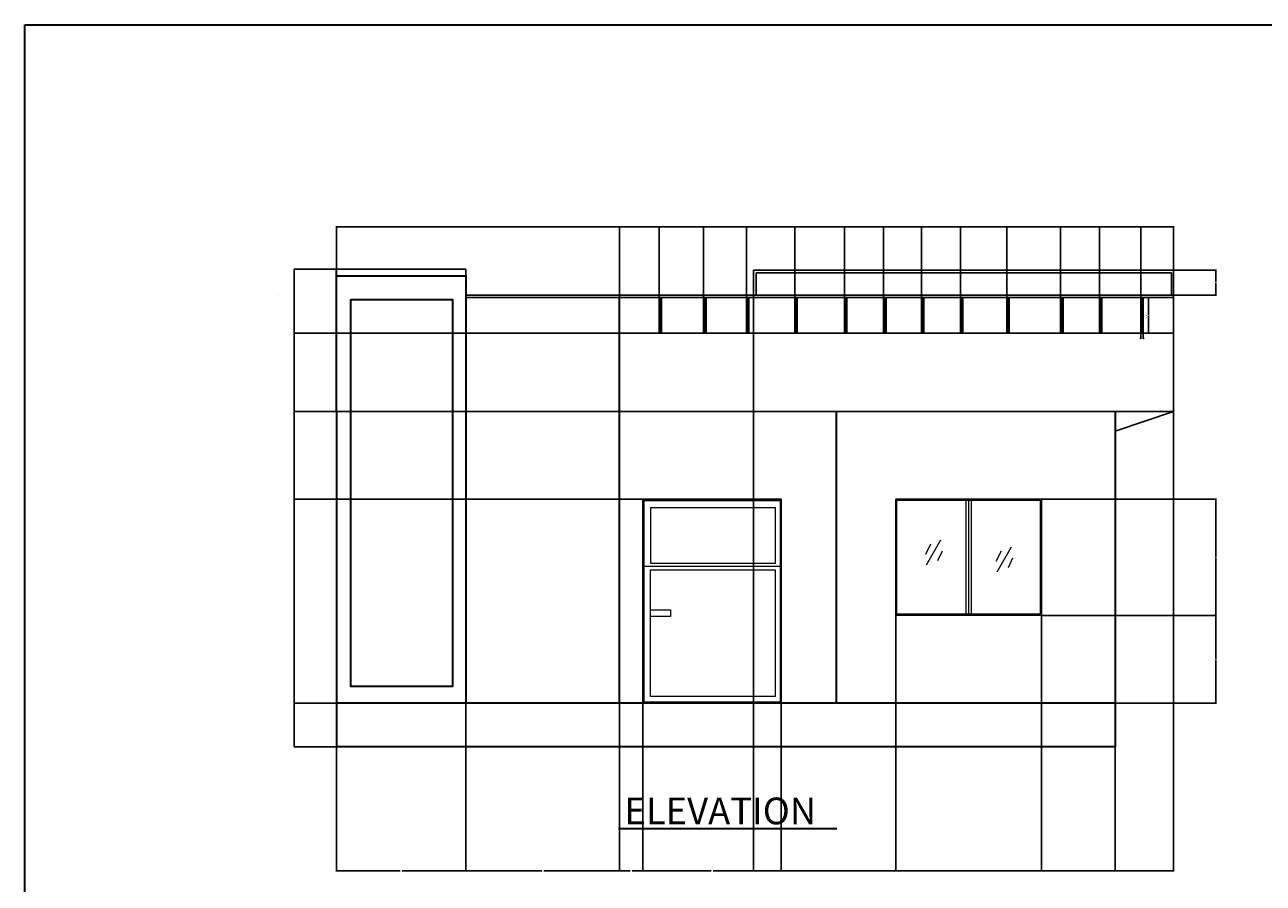
# Model space of a CAD drawing. Units: inches. Extents: x 1441 to 2460, y 1648 to 2683.
# Tile 34 of 35: x 1441 to 1950, y 2329 to 2683. Entities that reach past the tile are written whole.
import ezdxf

# ---------------------------------------------------------------- set-up
doc = ezdxf.new("R2010")
doc.units = ezdxf.units.IN
for name, color, linetype, lineweight in [('A-ANNO-DIMS', 2, 'Continuous', 18), ('A-ANNO-TITL', 7, 'Continuous', 30), ('A-ANNO-TTLB', 7, 'Continuous', 35), ('A-ELEV', 7, 'Continuous', 30), ('A-ELEV-DOOR', 3, 'Continuous', 20), ('A-ELEV-GLAZ', 4, 'Continuous', 18), ('A-ROOF', 7, 'Continuous', 25)]:
    doc.layers.add(name, color=color, linetype=linetype, lineweight=lineweight)
doc.styles.get("Standard").update_dxf_attribs({"font": 'arial.ttf'})
doc.dimstyles.get("Standard").update_dxf_attribs({"dimtxt": 0.18, "dimasz": 0.18, "dimexe": 0.18, "dimexo": 0.0625, "dimgap": 0.09, "dimtad": 0, "dimtih": 1, "dimtoh": 1, "dimdec": 4, "dimzin": 0, "dimdsep": 46, "dimtxsty": 'Standard', "dimcen": 0.09, "dimadec": 0, "dimazin": 0, "dimtfac": 1, "dimtdec": 4, "dimtofl": 0, "dimtmove": 0, "dimatfit": 3, "dimfxl": 1, "dimtolj": 1, "dimtzin": 0, "dimarcsym": 0})

# ---------------------------------------------------------------- blocks, each defined once
blk = doc.blocks.new('PARAPET-MULLION-ELEV')
for p, q in [((0, 14.7), (0, 0)), ((0.5, 0), (0.5, 14.7)), ((1, 14.7), (1, 0))]:
    blk.add_line(p, q)
blk = doc.blocks.new('*D64')
at = {"layer": 'A-ANNO-DIMS', "color": 0, "lineweight": -2, "transparency": 16777216}
for p, q in [((1900.97, 2570.36), (1903.29, 2570.36)), ((1903.11, 2570.18), (1903.11, 2563.2)), ((1903.11, 2555.84), (1903.11, 2562.83)), ((1900.97, 2555.66), (1903.29, 2555.66))]:
    blk.add_line(p, q, dxfattribs=at)
at = {"layer": 'A-ANNO-DIMS', "color": 0, "transparency": 16777216}
for points in [[(1903.08, 2570.18), (1903.14, 2570.18), (1903.11, 2570.36)], [(1903.08, 2555.84), (1903.14, 2555.84), (1903.11, 2555.66)]]:
    blk.add_solid(points, dxfattribs=at)
at = {"layer": 'Defpoints', "color": 0, "transparency": 16777216}
for p in [(1900.91, 2570.36), (1903.11, 2570.36), (1900.91, 2555.66)]:
    blk.add_point(p, dxfattribs=at)
at = {"layer": 'A-ANNO-DIMS', "color": 0, "transparency": 16777216, "insert": (1903.11, 2563.01), "char_height": 0.18, "attachment_point": 5}
blk.add_mtext('\\A1;MULLION 15 TYP.', dxfattribs=at)
blk = doc.blocks.new('*D65')
at = {"layer": 'A-ANNO-DIMS', "color": 0, "lineweight": -2, "transparency": 16777216}
for p, q in [((1899.91, 2555.6), (1899.91, 2553.28)), ((1900.91, 2555.6), (1900.91, 2553.28)), ((1899.73, 2553.46), (1899.55, 2553.46)), ((1901.09, 2553.46), (1901.27, 2553.46))]:
    blk.add_line(p, q, dxfattribs=at)
at = {"layer": 'A-ANNO-DIMS', "color": 0, "transparency": 16777216}
for points in [[(1899.73, 2553.49), (1899.73, 2553.43), (1899.91, 2553.46)], [(1901.09, 2553.49), (1901.09, 2553.43), (1900.91, 2553.46)]]:
    blk.add_solid(points, dxfattribs=at)
at = {"layer": 'Defpoints', "color": 0, "transparency": 16777216}
for p in [(1899.91, 2555.66), (1900.91, 2555.66), (1900.91, 2553.46)]:
    blk.add_point(p, dxfattribs=at)
at = {"layer": 'A-ANNO-DIMS', "color": 0, "transparency": 16777216, "insert": (1900.41, 2553.46), "char_height": 0.18, "attachment_point": 5}
blk.add_mtext('\\A1;1 TYP.', dxfattribs=at)
blk = doc.blocks.new('*D90')
at = {"layer": 'A-ANNO-DIMS', "color": 0, "lineweight": -2, "transparency": 16777216}
for p, q in [((1568.89, 2582.04), (1568.89, 2599.66)), ((1569.07, 2599.48), (1740.74, 2599.48)), ((1913.21, 2599.48), (1741.53, 2599.48)), ((1913.39, 2581.67), (1913.39, 2599.66))]:
    blk.add_line(p, q, dxfattribs=at)
at = {"layer": 'A-ANNO-DIMS', "color": 0, "transparency": 16777216}
for points in [[(1569.07, 2599.51), (1569.07, 2599.45), (1568.89, 2599.48)], [(1913.21, 2599.51), (1913.21, 2599.45), (1913.39, 2599.48)]]:
    blk.add_solid(points, dxfattribs=at)
at = {"layer": 'Defpoints', "color": 0, "transparency": 16777216}
for p in [(1913.39, 2599.48), (1568.89, 2581.98), (1913.39, 2581.61)]:
    blk.add_point(p, dxfattribs=at)
at = {"layer": 'A-ANNO-DIMS', "color": 0, "transparency": 16777216, "insert": (1741.14, 2599.48), "char_height": 0.18, "attachment_point": 5}
blk.add_mtext('\\A1;344.5', dxfattribs=at)
blk = doc.blocks.new('*D91')
at = {"layer": 'A-ANNO-DIMS', "color": 0, "lineweight": -2, "transparency": 16777216}
for p, q in [((1568.82, 2581.98), (1551.21, 2581.98)), ((1551.39, 2581.8), (1551.39, 2483.85)), ((1551.39, 2385.54), (1551.39, 2483.49)), ((1568.82, 2385.36), (1551.21, 2385.36))]:
    blk.add_line(p, q, dxfattribs=at)
at = {"layer": 'A-ANNO-DIMS', "color": 0, "transparency": 16777216}
for points in [[(1551.36, 2581.8), (1551.42, 2581.8), (1551.39, 2581.98)], [(1551.36, 2385.54), (1551.42, 2385.54), (1551.39, 2385.36)]]:
    blk.add_solid(points, dxfattribs=at)
at = {"layer": 'Defpoints', "color": 0, "transparency": 16777216}
for p in [(1551.39, 2581.98), (1568.89, 2581.98), (1568.89, 2385.36)]:
    blk.add_point(p, dxfattribs=at)
at = {"layer": 'A-ANNO-DIMS', "color": 0, "transparency": 16777216, "insert": (1551.39, 2483.67), "char_height": 0.18, "attachment_point": 5}
blk.add_mtext('\\A1;196.6', dxfattribs=at)
blk = doc.blocks.new('*D92')
at = {"layer": 'A-ANNO-DIMS', "color": 0, "lineweight": -2, "transparency": 16777216}
for p, q in [((1568.89, 2403.3), (1568.89, 2334.04)), ((1622.11, 2403.3), (1622.11, 2334.04)), ((1569.07, 2334.22), (1595.11, 2334.22)), ((1621.93, 2334.22), (1595.89, 2334.22))]:
    blk.add_line(p, q, dxfattribs=at)
at = {"layer": 'A-ANNO-DIMS', "color": 0, "transparency": 16777216}
for points in [[(1569.07, 2334.25), (1569.07, 2334.19), (1568.89, 2334.22)], [(1621.93, 2334.25), (1621.93, 2334.19), (1622.11, 2334.22)]]:
    blk.add_solid(points, dxfattribs=at)
at = {"layer": 'Defpoints', "color": 0, "transparency": 16777216}
for p in [(1568.89, 2403.36), (1622.11, 2403.36), (1622.11, 2334.22)]:
    blk.add_point(p, dxfattribs=at)
at = {"layer": 'A-ANNO-DIMS', "color": 0, "transparency": 16777216, "insert": (1595.5, 2334.22), "char_height": 0.18, "attachment_point": 5}
blk.add_mtext('\\A1;53.23', dxfattribs=at)
blk = doc.blocks.new('*D93')
at = {"layer": 'A-ANNO-DIMS', "color": 0, "lineweight": -2, "transparency": 16777216}
for p, q in [((1622.11, 2403.3), (1622.11, 2334.04)), ((1685.39, 2403.3), (1685.39, 2334.04)), ((1622.29, 2334.22), (1653.36, 2334.22)), ((1685.21, 2334.22), (1654.15, 2334.22))]:
    blk.add_line(p, q, dxfattribs=at)
at = {"layer": 'A-ANNO-DIMS', "color": 0, "transparency": 16777216}
for points in [[(1622.29, 2334.25), (1622.29, 2334.19), (1622.11, 2334.22)], [(1685.21, 2334.25), (1685.21, 2334.19), (1685.39, 2334.22)]]:
    blk.add_solid(points, dxfattribs=at)
at = {"layer": 'Defpoints', "color": 0, "transparency": 16777216}
for p in [(1622.11, 2403.36), (1685.39, 2403.36), (1685.39, 2334.22)]:
    blk.add_point(p, dxfattribs=at)
at = {"layer": 'A-ANNO-DIMS', "color": 0, "transparency": 16777216, "insert": (1653.75, 2334.22), "char_height": 0.18, "attachment_point": 5}
blk.add_mtext('\\A1;63.28', dxfattribs=at)
blk = doc.blocks.new('*D94')
at = {"layer": 'A-ANNO-DIMS', "color": 0, "lineweight": -2, "transparency": 16777216}
for p, q in [((1685.39, 2403.3), (1685.39, 2334.04)), ((1695, 2403.3), (1695, 2334.04)), ((1685.57, 2334.22), (1689.8, 2334.22)), ((1694.82, 2334.22), (1690.59, 2334.22))]:
    blk.add_line(p, q, dxfattribs=at)
at = {"layer": 'A-ANNO-DIMS', "color": 0, "transparency": 16777216}
for points in [[(1685.57, 2334.25), (1685.57, 2334.19), (1685.39, 2334.22)], [(1694.82, 2334.25), (1694.82, 2334.19), (1695, 2334.22)]]:
    blk.add_solid(points, dxfattribs=at)
at = {"layer": 'Defpoints', "color": 0, "transparency": 16777216}
for p in [(1685.39, 2403.36), (1695, 2403.36), (1695, 2334.22)]:
    blk.add_point(p, dxfattribs=at)
at = {"layer": 'A-ANNO-DIMS', "color": 0, "transparency": 16777216, "insert": (1690.2, 2334.22), "char_height": 0.18, "attachment_point": 5}
blk.add_mtext('\\A1;9.614', dxfattribs=at)
blk = doc.blocks.new('*D95')
at = {"layer": 'A-ANNO-DIMS', "color": 0, "lineweight": -2, "transparency": 16777216}
for p, q in [((1695, 2403.3), (1695, 2334.04)), ((1751.89, 2403.3), (1751.89, 2334.04)), ((1695.18, 2334.22), (1723.06, 2334.22)), ((1751.71, 2334.22), (1723.84, 2334.22))]:
    blk.add_line(p, q, dxfattribs=at)
at = {"layer": 'A-ANNO-DIMS', "color": 0, "transparency": 16777216}
for points in [[(1695.18, 2334.25), (1695.18, 2334.19), (1695, 2334.22)], [(1751.71, 2334.25), (1751.71, 2334.19), (1751.89, 2334.22)]]:
    blk.add_solid(points, dxfattribs=at)
at = {"layer": 'Defpoints', "color": 0, "transparency": 16777216}
for p in [(1695, 2403.36), (1751.89, 2403.36), (1751.89, 2334.22)]:
    blk.add_point(p, dxfattribs=at)
at = {"layer": 'A-ANNO-DIMS', "color": 0, "transparency": 16777216, "insert": (1723.45, 2334.22), "char_height": 0.18, "attachment_point": 5}
blk.add_mtext('\\A1;56.89', dxfattribs=at)
blk = doc.blocks.new('*D96')
at = {"layer": 'A-ANNO-DIMS', "color": 0, "lineweight": -2, "transparency": 16777216}
for p, q in [((1751.89, 2487.3), (1751.89, 2334.04)), ((1799.11, 2487.3), (1799.11, 2334.04)), ((1752.07, 2334.22), (1775.11, 2334.22)), ((1798.93, 2334.22), (1775.9, 2334.22))]:
    blk.add_line(p, q, dxfattribs=at)
at = {"layer": 'A-ANNO-DIMS', "color": 0, "transparency": 16777216}
for points in [[(1752.07, 2334.25), (1752.07, 2334.19), (1751.89, 2334.22)], [(1798.93, 2334.25), (1798.93, 2334.19), (1799.11, 2334.22)]]:
    blk.add_solid(points, dxfattribs=at)
at = {"layer": 'Defpoints', "color": 0, "transparency": 16777216}
for p in [(1751.89, 2487.36), (1799.11, 2487.36), (1799.11, 2334.22)]:
    blk.add_point(p, dxfattribs=at)
at = {"layer": 'A-ANNO-DIMS', "color": 0, "transparency": 16777216, "insert": (1775.5, 2334.22), "char_height": 0.18, "attachment_point": 5}
blk.add_mtext('\\A1;47.22', dxfattribs=at)
blk = doc.blocks.new('*D97')
at = {"layer": 'A-ANNO-DIMS', "color": 0, "lineweight": -2, "transparency": 16777216}
for p, q in [((1799.11, 2439.3), (1799.11, 2334.04)), ((1859.11, 2439.3), (1859.11, 2334.04)), ((1799.29, 2334.22), (1828.89, 2334.22)), ((1858.93, 2334.22), (1829.33, 2334.22))]:
    blk.add_line(p, q, dxfattribs=at)
at = {"layer": 'A-ANNO-DIMS', "color": 0, "transparency": 16777216}
for points in [[(1799.29, 2334.25), (1799.29, 2334.19), (1799.11, 2334.22)], [(1858.93, 2334.25), (1858.93, 2334.19), (1859.11, 2334.22)]]:
    blk.add_solid(points, dxfattribs=at)
at = {"layer": 'Defpoints', "color": 0, "transparency": 16777216}
for p in [(1799.11, 2439.36), (1859.11, 2439.36), (1859.11, 2334.22)]:
    blk.add_point(p, dxfattribs=at)
at = {"layer": 'A-ANNO-DIMS', "color": 0, "transparency": 16777216, "insert": (1829.11, 2334.22), "char_height": 0.18, "attachment_point": 5}
blk.add_mtext('\\A1;60', dxfattribs=at)
blk = doc.blocks.new('*D98')
at = {"layer": 'A-ANNO-DIMS', "color": 0, "lineweight": -2, "transparency": 16777216}
for p, q in [((1859.11, 2439.3), (1859.11, 2334.04)), ((1889.39, 2403.3), (1889.39, 2334.04)), ((1859.29, 2334.22), (1873.86, 2334.22)), ((1889.21, 2334.22), (1874.64, 2334.22))]:
    blk.add_line(p, q, dxfattribs=at)
at = {"layer": 'A-ANNO-DIMS', "color": 0, "transparency": 16777216}
for points in [[(1859.29, 2334.25), (1859.29, 2334.19), (1859.11, 2334.22)], [(1889.21, 2334.25), (1889.21, 2334.19), (1889.39, 2334.22)]]:
    blk.add_solid(points, dxfattribs=at)
at = {"layer": 'Defpoints', "color": 0, "transparency": 16777216}
for p in [(1859.11, 2439.36), (1889.39, 2403.36), (1889.39, 2334.22)]:
    blk.add_point(p, dxfattribs=at)
at = {"layer": 'A-ANNO-DIMS', "color": 0, "transparency": 16777216, "insert": (1874.25, 2334.22), "char_height": 0.18, "attachment_point": 5}
blk.add_mtext('\\A1;30.27', dxfattribs=at)
blk = doc.blocks.new('*D99')
at = {"layer": 'A-ANNO-DIMS', "color": 0, "lineweight": -2, "transparency": 16777216}
for p, q in [((1913.39, 2523.3), (1913.39, 2334.04)), ((1889.39, 2385.3), (1889.39, 2334.04)), ((1889.57, 2334.22), (1901.17, 2334.22)), ((1913.21, 2334.22), (1901.61, 2334.22))]:
    blk.add_line(p, q, dxfattribs=at)
at = {"layer": 'A-ANNO-DIMS', "color": 0, "transparency": 16777216}
for points in [[(1889.57, 2334.25), (1889.57, 2334.19), (1889.39, 2334.22)], [(1913.21, 2334.25), (1913.21, 2334.19), (1913.39, 2334.22)]]:
    blk.add_solid(points, dxfattribs=at)
at = {"layer": 'Defpoints', "color": 0, "transparency": 16777216}
for p in [(1913.39, 2523.36), (1889.39, 2385.36), (1913.39, 2334.22)]:
    blk.add_point(p, dxfattribs=at)
at = {"layer": 'A-ANNO-DIMS', "color": 0, "transparency": 16777216, "insert": (1901.39, 2334.22), "char_height": 0.18, "attachment_point": 5}
blk.add_mtext('\\A1;24', dxfattribs=at)
blk = doc.blocks.new('*D100')
at = {"layer": 'A-ANNO-DIMS', "color": 0, "lineweight": -2, "transparency": 16777216}
for p, q in [((1694.94, 2487.36), (1551.21, 2487.36)), ((1551.39, 2487.18), (1551.39, 2445.54)), ((1551.39, 2403.54), (1551.39, 2445.18)), ((1694.94, 2403.36), (1551.21, 2403.36))]:
    blk.add_line(p, q, dxfattribs=at)
at = {"layer": 'A-ANNO-DIMS', "color": 0, "transparency": 16777216}
for points in [[(1551.36, 2487.18), (1551.42, 2487.18), (1551.39, 2487.36)], [(1551.36, 2403.54), (1551.42, 2403.54), (1551.39, 2403.36)]]:
    blk.add_solid(points, dxfattribs=at)
at = {"layer": 'Defpoints', "color": 0, "transparency": 16777216}
for p in [(1551.39, 2487.36), (1695, 2487.36), (1695, 2403.36)]:
    blk.add_point(p, dxfattribs=at)
at = {"layer": 'A-ANNO-DIMS', "color": 0, "transparency": 16777216, "insert": (1551.39, 2445.36), "char_height": 0.18, "attachment_point": 5}
blk.add_mtext('\\A1;84', dxfattribs=at)
blk = doc.blocks.new('*D101')
at = {"layer": 'A-ANNO-DIMS', "color": 0, "lineweight": -2, "transparency": 16777216}
for p, q in [((1859.18, 2487.36), (1931.07, 2487.36)), ((1930.89, 2487.18), (1930.89, 2463.54)), ((1930.89, 2439.54), (1930.89, 2463.18)), ((1859.18, 2439.36), (1931.07, 2439.36))]:
    blk.add_line(p, q, dxfattribs=at)
at = {"layer": 'A-ANNO-DIMS', "color": 0, "transparency": 16777216}
for points in [[(1930.86, 2487.18), (1930.92, 2487.18), (1930.89, 2487.36)], [(1930.86, 2439.54), (1930.92, 2439.54), (1930.89, 2439.36)]]:
    blk.add_solid(points, dxfattribs=at)
at = {"layer": 'Defpoints', "color": 0, "transparency": 16777216}
for p in [(1859.11, 2487.36), (1930.89, 2487.36), (1859.11, 2439.36)]:
    blk.add_point(p, dxfattribs=at)
at = {"layer": 'A-ANNO-DIMS', "color": 0, "transparency": 16777216, "insert": (1930.89, 2463.36), "char_height": 0.18, "attachment_point": 5}
blk.add_mtext('\\A1;48', dxfattribs=at)
blk = doc.blocks.new('*D102')
at = {"layer": 'A-ANNO-DIMS', "color": 0, "lineweight": -2, "transparency": 16777216}
for p, q in [((1859.18, 2439.36), (1931.07, 2439.36)), ((1930.89, 2439.18), (1930.89, 2421.54)), ((1930.89, 2403.54), (1930.89, 2421.18)), ((1889.45, 2403.36), (1931.07, 2403.36))]:
    blk.add_line(p, q, dxfattribs=at)
at = {"layer": 'A-ANNO-DIMS', "color": 0, "transparency": 16777216}
for points in [[(1930.86, 2439.18), (1930.92, 2439.18), (1930.89, 2439.36)], [(1930.86, 2403.54), (1930.92, 2403.54), (1930.89, 2403.36)]]:
    blk.add_solid(points, dxfattribs=at)
at = {"layer": 'Defpoints', "color": 0, "transparency": 16777216}
for p in [(1859.11, 2439.36), (1889.39, 2403.36), (1930.89, 2403.36)]:
    blk.add_point(p, dxfattribs=at)
at = {"layer": 'A-ANNO-DIMS', "color": 0, "transparency": 16777216, "insert": (1930.89, 2421.36), "char_height": 0.18, "attachment_point": 5}
blk.add_mtext('\\A1;36', dxfattribs=at)
blk = doc.blocks.new('*D103')
at = {"layer": 'A-ANNO-DIMS', "color": 0, "lineweight": -2, "transparency": 16777216}
for p, q in [((1685.39, 2570.42), (1685.39, 2599.66)), ((1685.57, 2599.48), (1693.05, 2599.48)), ((1701.45, 2599.48), (1693.96, 2599.48)), ((1701.63, 2570.42), (1701.63, 2599.66))]:
    blk.add_line(p, q, dxfattribs=at)
at = {"layer": 'A-ANNO-DIMS', "color": 0, "transparency": 16777216}
for points in [[(1685.57, 2599.51), (1685.57, 2599.45), (1685.39, 2599.48)], [(1701.45, 2599.51), (1701.45, 2599.45), (1701.63, 2599.48)]]:
    blk.add_solid(points, dxfattribs=at)
at = {"layer": 'Defpoints', "color": 0, "transparency": 16777216}
for p in [(1701.63, 2599.48), (1685.39, 2570.36), (1701.63, 2570.36)]:
    blk.add_point(p, dxfattribs=at)
at = {"layer": 'A-ANNO-DIMS', "color": 0, "transparency": 16777216, "insert": (1693.51, 2599.48), "char_height": 0.18, "attachment_point": 5}
blk.add_mtext('\\A1;16.236', dxfattribs=at)
blk = doc.blocks.new('*D104')
at = {"layer": 'A-ANNO-DIMS', "color": 0, "lineweight": -2, "transparency": 16777216}
for p, q in [((1701.63, 2570.42), (1701.63, 2599.66)), ((1701.81, 2599.48), (1710.33, 2599.48)), ((1719.77, 2599.48), (1711.24, 2599.48)), ((1719.95, 2570.42), (1719.95, 2599.66))]:
    blk.add_line(p, q, dxfattribs=at)
at = {"layer": 'A-ANNO-DIMS', "color": 0, "transparency": 16777216}
for points in [[(1701.81, 2599.51), (1701.81, 2599.45), (1701.63, 2599.48)], [(1719.77, 2599.51), (1719.77, 2599.45), (1719.95, 2599.48)]]:
    blk.add_solid(points, dxfattribs=at)
at = {"layer": 'Defpoints', "color": 0, "transparency": 16777216}
for p in [(1719.95, 2599.48), (1701.63, 2570.36), (1719.95, 2570.36)]:
    blk.add_point(p, dxfattribs=at)
at = {"layer": 'A-ANNO-DIMS', "color": 0, "transparency": 16777216, "insert": (1710.79, 2599.48), "char_height": 0.18, "attachment_point": 5}
blk.add_mtext('\\A1;18.327', dxfattribs=at)
blk = doc.blocks.new('*D105')
at = {"layer": 'A-ANNO-DIMS', "color": 0, "lineweight": -2, "transparency": 16777216}
for p, q in [((1719.95, 2570.42), (1719.95, 2599.66)), ((1720.13, 2599.48), (1728.3, 2599.48)), ((1737.38, 2599.48), (1729.21, 2599.48)), ((1737.56, 2570.42), (1737.56, 2599.66))]:
    blk.add_line(p, q, dxfattribs=at)
at = {"layer": 'A-ANNO-DIMS', "color": 0, "transparency": 16777216}
for points in [[(1720.13, 2599.51), (1720.13, 2599.45), (1719.95, 2599.48)], [(1737.38, 2599.51), (1737.38, 2599.45), (1737.56, 2599.48)]]:
    blk.add_solid(points, dxfattribs=at)
at = {"layer": 'Defpoints', "color": 0, "transparency": 16777216}
for p in [(1737.56, 2599.48), (1719.95, 2570.36), (1737.56, 2570.36)]:
    blk.add_point(p, dxfattribs=at)
at = {"layer": 'A-ANNO-DIMS', "color": 0, "transparency": 16777216, "insert": (1728.76, 2599.48), "char_height": 0.18, "attachment_point": 5}
blk.add_mtext('\\A1;17.604', dxfattribs=at)
blk = doc.blocks.new('*D106')
at = {"layer": 'A-ANNO-DIMS', "color": 0, "lineweight": -2, "transparency": 16777216}
for p, q in [((1737.56, 2570.42), (1737.56, 2599.66)), ((1737.74, 2599.48), (1747.15, 2599.48)), ((1757.33, 2599.48), (1747.92, 2599.48)), ((1757.51, 2570.42), (1757.51, 2599.66))]:
    blk.add_line(p, q, dxfattribs=at)
at = {"layer": 'A-ANNO-DIMS', "color": 0, "transparency": 16777216}
for points in [[(1737.74, 2599.51), (1737.74, 2599.45), (1737.56, 2599.48)], [(1757.33, 2599.51), (1757.33, 2599.45), (1757.51, 2599.48)]]:
    blk.add_solid(points, dxfattribs=at)
at = {"layer": 'Defpoints', "color": 0, "transparency": 16777216}
for p in [(1757.51, 2599.48), (1737.56, 2570.36), (1757.51, 2570.36)]:
    blk.add_point(p, dxfattribs=at)
at = {"layer": 'A-ANNO-DIMS', "color": 0, "transparency": 16777216, "insert": (1747.53, 2599.48), "char_height": 0.18, "attachment_point": 5}
blk.add_mtext('\\A1;19.95', dxfattribs=at)
blk = doc.blocks.new('*D107')
at = {"layer": 'A-ANNO-DIMS', "color": 0, "lineweight": -2, "transparency": 16777216}
for p, q in [((1757.51, 2570.42), (1757.51, 2599.66)), ((1757.69, 2599.48), (1767.25, 2599.48)), ((1777.73, 2599.48), (1768.18, 2599.48)), ((1777.91, 2570.42), (1777.91, 2599.66))]:
    blk.add_line(p, q, dxfattribs=at)
at = {"layer": 'A-ANNO-DIMS', "color": 0, "transparency": 16777216}
for points in [[(1757.69, 2599.51), (1757.69, 2599.45), (1757.51, 2599.48)], [(1777.73, 2599.51), (1777.73, 2599.45), (1777.91, 2599.48)]]:
    blk.add_solid(points, dxfattribs=at)
at = {"layer": 'Defpoints', "color": 0, "transparency": 16777216}
for p in [(1777.91, 2599.48), (1757.51, 2570.36), (1777.91, 2570.36)]:
    blk.add_point(p, dxfattribs=at)
at = {"layer": 'A-ANNO-DIMS', "color": 0, "transparency": 16777216, "insert": (1767.71, 2599.48), "char_height": 0.18, "attachment_point": 5}
blk.add_mtext('\\A1;20.405', dxfattribs=at)
blk = doc.blocks.new('*D108')
at = {"layer": 'A-ANNO-DIMS', "color": 0, "lineweight": -2, "transparency": 16777216}
for p, q in [((1777.91, 2570.42), (1777.91, 2599.66)), ((1778.09, 2599.48), (1785.55, 2599.48)), ((1793.91, 2599.48), (1786.46, 2599.48)), ((1794.09, 2570.42), (1794.09, 2599.66))]:
    blk.add_line(p, q, dxfattribs=at)
at = {"layer": 'A-ANNO-DIMS', "color": 0, "transparency": 16777216}
for points in [[(1778.09, 2599.51), (1778.09, 2599.45), (1777.91, 2599.48)], [(1793.91, 2599.51), (1793.91, 2599.45), (1794.09, 2599.48)]]:
    blk.add_solid(points, dxfattribs=at)
at = {"layer": 'Defpoints', "color": 0, "transparency": 16777216}
for p in [(1794.09, 2599.48), (1777.91, 2570.36), (1794.09, 2570.36)]:
    blk.add_point(p, dxfattribs=at)
at = {"layer": 'A-ANNO-DIMS', "color": 0, "transparency": 16777216, "insert": (1786, 2599.48), "char_height": 0.18, "attachment_point": 5}
blk.add_mtext('\\A1;16.173', dxfattribs=at)
blk = doc.blocks.new('*D109')
at = {"layer": 'A-ANNO-DIMS', "color": 0, "lineweight": -2, "transparency": 16777216}
for p, q in [((1794.09, 2570.42), (1794.09, 2599.66)), ((1794.27, 2599.48), (1801.41, 2599.48)), ((1809.46, 2599.48), (1802.32, 2599.48)), ((1809.64, 2570.42), (1809.64, 2599.66))]:
    blk.add_line(p, q, dxfattribs=at)
at = {"layer": 'A-ANNO-DIMS', "color": 0, "transparency": 16777216}
for points in [[(1794.27, 2599.51), (1794.27, 2599.45), (1794.09, 2599.48)], [(1809.46, 2599.51), (1809.46, 2599.45), (1809.64, 2599.48)]]:
    blk.add_solid(points, dxfattribs=at)
at = {"layer": 'Defpoints', "color": 0, "transparency": 16777216}
for p in [(1809.64, 2599.48), (1794.09, 2570.36), (1809.64, 2570.36)]:
    blk.add_point(p, dxfattribs=at)
at = {"layer": 'A-ANNO-DIMS', "color": 0, "transparency": 16777216, "insert": (1801.86, 2599.48), "char_height": 0.18, "attachment_point": 5}
blk.add_mtext('\\A1;15.554', dxfattribs=at)
blk = doc.blocks.new('*D110')
at = {"layer": 'A-ANNO-DIMS', "color": 0, "lineweight": -2, "transparency": 16777216}
for p, q in [((1809.64, 2570.42), (1809.64, 2599.66)), ((1809.82, 2599.48), (1817.2, 2599.48)), ((1825.49, 2599.48), (1818.11, 2599.48)), ((1825.67, 2570.42), (1825.67, 2599.66))]:
    blk.add_line(p, q, dxfattribs=at)
at = {"layer": 'A-ANNO-DIMS', "color": 0, "transparency": 16777216}
for points in [[(1809.82, 2599.51), (1809.82, 2599.45), (1809.64, 2599.48)], [(1825.49, 2599.51), (1825.49, 2599.45), (1825.67, 2599.48)]]:
    blk.add_solid(points, dxfattribs=at)
at = {"layer": 'Defpoints', "color": 0, "transparency": 16777216}
for p in [(1825.67, 2599.48), (1809.64, 2570.36), (1825.67, 2570.36)]:
    blk.add_point(p, dxfattribs=at)
at = {"layer": 'A-ANNO-DIMS', "color": 0, "transparency": 16777216, "insert": (1817.65, 2599.48), "char_height": 0.18, "attachment_point": 5}
blk.add_mtext('\\A1;16.025', dxfattribs=at)
blk = doc.blocks.new('*D111')
at = {"layer": 'A-ANNO-DIMS', "color": 0, "lineweight": -2, "transparency": 16777216}
for p, q in [((1825.67, 2570.42), (1825.67, 2599.66)), ((1825.85, 2599.48), (1834.75, 2599.48)), ((1844.56, 2599.48), (1835.66, 2599.48)), ((1844.74, 2570.42), (1844.74, 2599.66))]:
    blk.add_line(p, q, dxfattribs=at)
at = {"layer": 'A-ANNO-DIMS', "color": 0, "transparency": 16777216}
for points in [[(1825.85, 2599.51), (1825.85, 2599.45), (1825.67, 2599.48)], [(1844.56, 2599.51), (1844.56, 2599.45), (1844.74, 2599.48)]]:
    blk.add_solid(points, dxfattribs=at)
at = {"layer": 'Defpoints', "color": 0, "transparency": 16777216}
for p in [(1844.74, 2599.48), (1825.67, 2570.36), (1844.74, 2570.36)]:
    blk.add_point(p, dxfattribs=at)
at = {"layer": 'A-ANNO-DIMS', "color": 0, "transparency": 16777216, "insert": (1835.2, 2599.48), "char_height": 0.18, "attachment_point": 5}
blk.add_mtext('\\A1;19.074', dxfattribs=at)
blk = doc.blocks.new('*D112')
at = {"layer": 'A-ANNO-DIMS', "color": 0, "lineweight": -2, "transparency": 16777216}
for p, q in [((1844.74, 2570.42), (1844.74, 2599.66)), ((1844.92, 2599.48), (1855.37, 2599.48)), ((1866.74, 2599.48), (1856.3, 2599.48)), ((1866.92, 2570.42), (1866.92, 2599.66))]:
    blk.add_line(p, q, dxfattribs=at)
at = {"layer": 'A-ANNO-DIMS', "color": 0, "transparency": 16777216}
for points in [[(1844.92, 2599.51), (1844.92, 2599.45), (1844.74, 2599.48)], [(1866.74, 2599.51), (1866.74, 2599.45), (1866.92, 2599.48)]]:
    blk.add_solid(points, dxfattribs=at)
at = {"layer": 'Defpoints', "color": 0, "transparency": 16777216}
for p in [(1866.92, 2599.48), (1844.74, 2570.36), (1866.92, 2570.36)]:
    blk.add_point(p, dxfattribs=at)
at = {"layer": 'A-ANNO-DIMS', "color": 0, "transparency": 16777216, "insert": (1855.83, 2599.48), "char_height": 0.18, "attachment_point": 5}
blk.add_mtext('\\A1;22.184', dxfattribs=at)
blk = doc.blocks.new('*D113')
at = {"layer": 'A-ANNO-DIMS', "color": 0, "lineweight": -2, "transparency": 16777216}
for p, q in [((1866.92, 2570.42), (1866.92, 2599.66)), ((1867.1, 2599.48), (1874.46, 2599.48)), ((1882.73, 2599.48), (1875.37, 2599.48)), ((1882.91, 2570.42), (1882.91, 2599.66))]:
    blk.add_line(p, q, dxfattribs=at)
at = {"layer": 'A-ANNO-DIMS', "color": 0, "transparency": 16777216}
for points in [[(1867.1, 2599.51), (1867.1, 2599.45), (1866.92, 2599.48)], [(1882.73, 2599.51), (1882.73, 2599.45), (1882.91, 2599.48)]]:
    blk.add_solid(points, dxfattribs=at)
at = {"layer": 'Defpoints', "color": 0, "transparency": 16777216}
for p in [(1882.91, 2599.48), (1866.92, 2570.36), (1882.91, 2570.36)]:
    blk.add_point(p, dxfattribs=at)
at = {"layer": 'A-ANNO-DIMS', "color": 0, "transparency": 16777216, "insert": (1874.92, 2599.48), "char_height": 0.18, "attachment_point": 5}
blk.add_mtext('\\A1;15.987', dxfattribs=at)
blk = doc.blocks.new('*D114')
at = {"layer": 'A-ANNO-DIMS', "color": 0, "lineweight": -2, "transparency": 16777216}
for p, q in [((1882.91, 2570.42), (1882.91, 2599.66)), ((1883.09, 2599.48), (1890.95, 2599.48)), ((1899.73, 2599.48), (1891.86, 2599.48)), ((1899.91, 2570.42), (1899.91, 2599.66))]:
    blk.add_line(p, q, dxfattribs=at)
at = {"layer": 'A-ANNO-DIMS', "color": 0, "transparency": 16777216}
for points in [[(1883.09, 2599.51), (1883.09, 2599.45), (1882.91, 2599.48)], [(1899.73, 2599.51), (1899.73, 2599.45), (1899.91, 2599.48)]]:
    blk.add_solid(points, dxfattribs=at)
at = {"layer": 'Defpoints', "color": 0, "transparency": 16777216}
for p in [(1899.91, 2599.48), (1882.91, 2570.36), (1899.91, 2570.36)]:
    blk.add_point(p, dxfattribs=at)
at = {"layer": 'A-ANNO-DIMS', "color": 0, "transparency": 16777216, "insert": (1891.41, 2599.48), "char_height": 0.18, "attachment_point": 5}
blk.add_mtext('\\A1;16.997', dxfattribs=at)
blk = doc.blocks.new('*D115')
at = {"layer": 'A-ANNO-DIMS', "color": 0, "lineweight": -2, "transparency": 16777216}
for p, q in [((1899.91, 2570.42), (1899.91, 2599.66)), ((1900.09, 2599.48), (1906.19, 2599.48)), ((1913.21, 2599.48), (1907.1, 2599.48)), ((1913.39, 2570.42), (1913.39, 2599.66))]:
    blk.add_line(p, q, dxfattribs=at)
at = {"layer": 'A-ANNO-DIMS', "color": 0, "transparency": 16777216}
for points in [[(1900.09, 2599.51), (1900.09, 2599.45), (1899.91, 2599.48)], [(1913.21, 2599.51), (1913.21, 2599.45), (1913.39, 2599.48)]]:
    blk.add_solid(points, dxfattribs=at)
at = {"layer": 'Defpoints', "color": 0, "transparency": 16777216}
for p in [(1913.39, 2599.48), (1899.91, 2570.36), (1913.39, 2570.36)]:
    blk.add_point(p, dxfattribs=at)
at = {"layer": 'A-ANNO-DIMS', "color": 0, "transparency": 16777216, "insert": (1906.65, 2599.48), "char_height": 0.18, "attachment_point": 5}
blk.add_mtext('\\A1;13.478', dxfattribs=at)
blk = doc.blocks.new('*D116')
at = {"layer": 'A-ANNO-DIMS', "color": 0, "lineweight": -2, "transparency": 16777216}
for p, q in [((1685.33, 2555.66), (1551.21, 2555.66)), ((1551.39, 2555.48), (1551.39, 2539.69)), ((1551.39, 2523.54), (1551.39, 2539.33)), ((1685.33, 2523.36), (1551.21, 2523.36))]:
    blk.add_line(p, q, dxfattribs=at)
at = {"layer": 'A-ANNO-DIMS', "color": 0, "transparency": 16777216}
for points in [[(1551.36, 2555.48), (1551.42, 2555.48), (1551.39, 2555.66)], [(1551.36, 2523.54), (1551.42, 2523.54), (1551.39, 2523.36)]]:
    blk.add_solid(points, dxfattribs=at)
at = {"layer": 'Defpoints', "color": 0, "transparency": 16777216}
for p in [(1551.39, 2555.66), (1685.39, 2555.66), (1685.39, 2523.36)]:
    blk.add_point(p, dxfattribs=at)
at = {"layer": 'A-ANNO-DIMS', "color": 0, "transparency": 16777216, "insert": (1551.39, 2539.51), "char_height": 0.18, "attachment_point": 5}
blk.add_mtext('\\A1;32.3', dxfattribs=at)
blk = doc.blocks.new('*D117')
at = {"layer": 'A-ANNO-DIMS', "color": 0, "lineweight": -2, "transparency": 16777216}
for p, q in [((1913.45, 2581.61), (1931.07, 2581.61)), ((1930.89, 2581.43), (1930.89, 2576.67)), ((1930.89, 2571.54), (1930.89, 2576.3)), ((1913.45, 2571.36), (1931.07, 2571.36))]:
    blk.add_line(p, q, dxfattribs=at)
at = {"layer": 'A-ANNO-DIMS', "color": 0, "transparency": 16777216}
for points in [[(1930.86, 2581.43), (1930.92, 2581.43), (1930.89, 2581.61)], [(1930.86, 2571.54), (1930.92, 2571.54), (1930.89, 2571.36)]]:
    blk.add_solid(points, dxfattribs=at)
at = {"layer": 'Defpoints', "color": 0, "transparency": 16777216}
for p in [(1913.39, 2581.61), (1930.89, 2581.61), (1913.39, 2571.36)]:
    blk.add_point(p, dxfattribs=at)
at = {"layer": 'A-ANNO-DIMS', "color": 0, "transparency": 16777216, "insert": (1930.89, 2576.48), "char_height": 0.18, "attachment_point": 5}
blk.add_mtext('\\A1;10.244', dxfattribs=at)
blk = doc.blocks.new('*D118')
at = {"layer": 'A-ANNO-DIMS', "color": 0, "lineweight": -2, "transparency": 16777216}
for p, q in [((1740.45, 2571.3), (1740.45, 2334.04)), ((1913.39, 2523.3), (1913.39, 2334.04)), ((1740.63, 2334.22), (1826.46, 2334.22)), ((1913.21, 2334.22), (1827.37, 2334.22))]:
    blk.add_line(p, q, dxfattribs=at)
at = {"layer": 'A-ANNO-DIMS', "color": 0, "transparency": 16777216}
for points in [[(1740.63, 2334.25), (1740.63, 2334.19), (1740.45, 2334.22)], [(1913.21, 2334.25), (1913.21, 2334.19), (1913.39, 2334.22)]]:
    blk.add_solid(points, dxfattribs=at)
at = {"layer": 'Defpoints', "color": 0, "transparency": 16777216}
for p in [(1740.45, 2571.36), (1913.39, 2523.36), (1913.39, 2334.22)]:
    blk.add_point(p, dxfattribs=at)
at = {"layer": 'A-ANNO-DIMS', "color": 0, "transparency": 16777216, "insert": (1826.92, 2334.22), "char_height": 0.18, "attachment_point": 5}
blk.add_mtext('\\A1;172.94', dxfattribs=at)

msp = doc.modelspace()

# ---------------------------------------------------------------- linework, layer by layer
at = {"layer": 'A-ANNO-TITL'}
msp.add_line((1684.8664, 2351.7233), (1774.7859, 2351.7233), dxfattribs=at)
at = {"layer": 'A-ANNO-TTLB'}
msp.add_lwpolyline([(1440.5107, 2682.6413), (2460.193, 2682.6413), (2460.193, 1648.08), (1440.5107, 1648.08)], close=True, dxfattribs=at)
at = {"layer": 'A-ELEV'}
for p, q in [((1568.8859, 2523.3623), (1568.8859, 2581.9803)), ((1568.8859, 2579.3069), (1622.1131, 2579.3069)), ((1622.1131, 2579.3069), (1622.1131, 2403.3623)), ((1685.3898, 2403.3623), (1685.3898, 2570.3623)), ((1568.8859, 2523.3623), (1568.8859, 2385.3623)), ((1774.4729, 2523.3623), (1774.4729, 2403.3623)), ((1889.3859, 2523.3623), (1889.3859, 2385.3623)), ((1889.3859, 2403.3623), (1568.8859, 2403.3623)), ((1889.3859, 2385.3623), (1568.8859, 2385.3623))]:
    msp.add_line(p, q, dxfattribs=at)
msp.add_lwpolyline([(1574.7104, 2569.5248), (1616.5893, 2569.5248), (1616.5893, 2410.1722), (1574.7104, 2410.1722)], close=True, dxfattribs=at)
at = {"layer": 'A-ELEV-DOOR'}
for p, q in [((1695.0034, 2487.3623), (1695.0034, 2403.3623)), ((1751.8944, 2487.3623), (1695.0034, 2487.3623)), ((1751.8944, 2487.3623), (1751.8944, 2403.3623)), ((1695.5671, 2459.6989), (1751.5069, 2459.6989))]:
    msp.add_line(p, q, dxfattribs=at)
for points in [[(1695.0034, 2487.3623), (1751.8944, 2487.3623), (1751.8944, 2403.3623), (1695.0034, 2403.3623)], [(1695.5671, 2486.807), (1751.5069, 2486.807), (1751.5069, 2403.7318), (1695.5671, 2403.7318)], [(1698.255, 2483.7995), (1749.4822, 2483.7995), (1749.4822, 2460.8319), (1698.255, 2460.8319)], [(1698.168, 2458.2266), (1749.4334, 2458.2266), (1749.4334, 2406.0881), (1698.168, 2406.0881)], [(1698.168, 2441.7533), (1706.4026, 2441.7533), (1706.4026, 2439.0358), (1698.168, 2439.0358)]]:
    msp.add_lwpolyline(points, close=True, dxfattribs=at)
at = {"layer": 'A-ELEV-GLAZ'}
for p, q in [((1859.1136, 2487.3623), (1799.1136, 2487.3623)), ((1799.1136, 2487.3623), (1799.1136, 2439.3623)), ((1828.0613, 2439.8928), (1828.0613, 2486.9034)), ((1828.0613, 2486.9034), (1829.0613, 2486.9034)), ((1829.0613, 2486.9034), (1829.0613, 2439.8928)), ((1829.0613, 2486.9034), (1830.0613, 2486.9034)), ((1830.0613, 2486.9034), (1830.0613, 2439.8928)), ((1859.1136, 2487.3623), (1859.1136, 2439.3623)), ((1813.3924, 2468.8077), (1811.2678, 2464.5603)), ((1817.5485, 2470.3822), (1811.6448, 2460.072)), ((1818.1514, 2465.877), (1816.2818, 2461.8845)), ((1842.4142, 2465.9195), (1840.2896, 2461.6721)), ((1846.5704, 2467.494), (1840.6667, 2457.1837)), ((1847.1733, 2462.9888), (1845.3037, 2458.9962)), ((1859.1136, 2439.3623), (1799.1136, 2439.3623)), ((1829.0613, 2439.8928), (1828.0613, 2439.8928))]:
    msp.add_line(p, q, dxfattribs=at)
msp.add_lwpolyline([(1799.55, 2486.9034), (1858.5725, 2486.9034), (1858.5725, 2439.8928), (1799.55, 2439.8928)], close=True, dxfattribs=at)
at = {"layer": 'A-ROOF'}
for p, q in [((1568.8859, 2581.9803), (1622.1131, 2581.9803)), ((1622.1131, 2581.9803), (1622.1131, 2571.3623)), ((1913.3859, 2581.6067), (1740.4464, 2581.6067)), ((1740.4464, 2581.6067), (1740.4464, 2571.3623)), ((1741.5398, 2571.3623), (1741.5398, 2580.4699)), ((1741.5398, 2580.4699), (1912.6405, 2580.4699)), ((1912.6405, 2580.4699), (1912.6405, 2571.3623)), ((1913.3859, 2571.3623), (1913.3859, 2581.6067)), ((1544.8859, 2571.3623), (1544.8859, 2571.3623)), ((1913.3859, 2571.3623), (1622.1131, 2571.3623)), ((1622.1131, 2571.3623), (1622.1131, 2570.3623)), ((1622.1131, 2571.3623), (1622.1131, 2570.3623)), ((1622.1131, 2570.3623), (1913.3859, 2570.3623)), ((1640.8471, 2570.3623), (1641.3471, 2570.3623)), ((1913.3859, 2523.3623), (1913.3859, 2571.3623)), ((1685.3898, 2555.6616), (1913.3859, 2555.6616)), ((1913.3859, 2523.3623), (1685.3898, 2523.3623)), ((1913.3859, 2523.3623), (1889.3859, 2515.2631))]:
    msp.add_line(p, q, dxfattribs=at)

# ---------------------------------------------------------------- block references
for p in [(1701.63, 2555.66), (1719.9565, 2555.66), (1737.561, 2555.66), (1757.5124, 2555.66), (1777.9179, 2555.66), (1794.0907, 2555.66), (1809.6442, 2555.66), (1825.6692, 2555.66), (1844.7431, 2555.66), (1866.9274, 2555.66), (1882.9148, 2555.66), (1899.9116, 2555.66)]:
    msp.add_blockref('PARAPET-MULLION-ELEV', p, dxfattribs=at)

# ---------------------------------------------------------------- texts
at = {"layer": 'A-ANNO-TITL', "insert": (1687.3601, 2364.4159), "char_height": 11, "attachment_point": 1}
msp.add_mtext_dynamic_manual_height_columns('ELEVATION', width=235.390969, gutter_width=12.5, heights=[0], dxfattribs=at)

# ---------------------------------------------------------------- dimensions: what is measured, and where the dimension line sits
at = {"layer": 'A-ANNO-DIMS'}
for base, p1, p2, override, picture, middle in [((1913.3859, 2599.4803), (1568.8859, 2581.9803), (1913.3859, 2581.6067), {"dimdec": 1, "dimlfac": 1, "dimrnd": 0, "dimzin": 0, "dimdsep": 46, "dimlunit": 2}, '*D90', (1741.1359, 2599.4803)), ((1701.62625, 2599.48026), (1685.3898, 2570.36227), (1701.62625, 2570.36227), {"dimdec": 3, "dimlfac": 1, "dimrnd": 0, "dimzin": 0, "dimdsep": 46, "dimlunit": 2}, '*D103', (1693.50803, 2599.48026)), ((1719.9528, 2599.48026), (1701.62625, 2570.36227), (1719.9528, 2570.36227), {"dimdec": 3, "dimlfac": 1, "dimrnd": 0, "dimzin": 0, "dimdsep": 46, "dimlunit": 2}, '*D104', (1710.78953, 2599.48026)), ((1737.5572, 2599.4803), (1719.9528, 2570.3623), (1737.5572, 2570.3623), {"dimdec": 3, "dimlfac": 1, "dimrnd": 0, "dimzin": 0, "dimdsep": 46, "dimlunit": 2}, '*D105', (1728.755, 2599.4803)), ((1757.5087, 2599.4803), (1737.5572, 2570.3623), (1757.5087, 2570.3623), {"dimdec": 2, "dimlfac": 1, "dimrnd": 0, "dimzin": 0, "dimdsep": 46, "dimlunit": 2}, '*D106', (1747.533, 2599.4803)), ((1777.91417, 2599.480261), (1757.508673, 2570.362267), (1777.91417, 2570.362267), {"dimdec": 3, "dimlfac": 1, "dimrnd": 0, "dimzin": 0, "dimdsep": 46, "dimlunit": 2}, '*D107', (1767.711421, 2599.480261)), ((1794.0869, 2599.4803), (1777.9142, 2570.3623), (1794.0869, 2570.3623), {"dimdec": 3, "dimlfac": 1, "dimrnd": 0, "dimzin": 0, "dimdsep": 46, "dimlunit": 2}, '*D108', (1786.0005, 2599.4803)), ((1809.6405, 2599.4803), (1794.0869, 2570.3623), (1809.6405, 2570.3623), {"dimdec": 3, "dimlfac": 1, "dimrnd": 0, "dimzin": 0, "dimdsep": 46, "dimlunit": 2}, '*D109', (1801.8637, 2599.4803)), ((1825.6655, 2599.4803), (1809.6405, 2570.3623), (1825.6655, 2570.3623), {"dimdec": 3, "dimlfac": 1, "dimrnd": 0, "dimzin": 0, "dimdsep": 46, "dimlunit": 2}, '*D110', (1817.653, 2599.4803)), ((1844.7394, 2599.4803), (1825.6655, 2570.3623), (1844.7394, 2570.3623), {"dimdec": 3, "dimlfac": 1, "dimrnd": 0, "dimzin": 0, "dimdsep": 46, "dimlunit": 2}, '*D111', (1835.2024, 2599.4803)), ((1866.9236, 2599.4803), (1844.7394, 2570.3623), (1866.9236, 2570.3623), {"dimdec": 3, "dimlfac": 1, "dimrnd": 0, "dimzin": 0, "dimdsep": 46, "dimlunit": 2}, '*D112', (1855.8315, 2599.4803)), ((1882.91106, 2599.48026), (1866.92365, 2570.36227), (1882.91106, 2570.36227), {"dimdec": 3, "dimlfac": 1, "dimrnd": 0, "dimzin": 0, "dimdsep": 46, "dimlunit": 2}, '*D113', (1874.91736, 2599.48026)), ((1899.9078, 2599.4803), (1882.9111, 2570.3623), (1899.9078, 2570.3623), {"dimdec": 3, "dimlfac": 1, "dimrnd": 0, "dimzin": 0, "dimdsep": 46, "dimlunit": 2}, '*D114', (1891.4095, 2599.4803)), ((1913.3859, 2599.4803), (1899.9078, 2570.3623), (1913.3859, 2570.3623), {"dimdec": 3, "dimlfac": 1, "dimrnd": 0, "dimzin": 0, "dimdsep": 46, "dimlunit": 2}, '*D115', (1906.6469, 2599.4803)), ((1913.3859, 2334.2233), (1740.4464, 2571.3623), (1913.3859, 2523.3623), {"dimdec": 2, "dimlfac": 1, "dimrnd": 0, "dimzin": 0, "dimdsep": 46, "dimlunit": 2}, '*D118', (1826.9162, 2334.2233)), ((1913.3859, 2334.2233), (1889.3859, 2385.3623), (1913.3859, 2523.3623), {"dimdec": 0, "dimlfac": 1, "dimrnd": 0, "dimzin": 0, "dimdsep": 46, "dimlunit": 2}, '*D99', (1901.3859, 2334.2233)), ((1799.1136, 2334.2233), (1751.8944, 2487.3623), (1799.1136, 2487.3623), {"dimdec": 2, "dimlfac": 1, "dimrnd": 0, "dimzin": 0, "dimdsep": 46, "dimlunit": 2}, '*D96', (1775.504, 2334.2233)), ((1859.1136, 2334.2233), (1799.1136, 2439.3623), (1859.1136, 2439.3623), {"dimdec": 0, "dimlfac": 1, "dimrnd": 0, "dimzin": 0, "dimdsep": 46, "dimlunit": 2}, '*D97', (1829.1136, 2334.2233)), ((1889.3859, 2334.2233), (1859.1136, 2439.3623), (1889.3859, 2403.3623), {"dimdec": 2, "dimlfac": 1, "dimrnd": 0, "dimzin": 0, "dimdsep": 46, "dimlunit": 2}, '*D98', (1874.2497, 2334.2233)), ((1622.1131, 2334.2233), (1568.8859, 2403.3623), (1622.1131, 2403.3623), {"dimdec": 2, "dimlfac": 1, "dimrnd": 0, "dimzin": 0, "dimdsep": 46, "dimlunit": 2}, '*D92', (1595.4995, 2334.2233)), ((1685.3898, 2334.2233), (1622.1131, 2403.3623), (1685.3898, 2403.3623), {"dimdec": 2, "dimlfac": 1, "dimrnd": 0, "dimzin": 0, "dimdsep": 46, "dimlunit": 2}, '*D93', (1653.7514, 2334.2233)), ((1695.0034, 2334.2233), (1685.3898, 2403.3623), (1695.0034, 2403.3623), {"dimdec": 3, "dimlfac": 1, "dimrnd": 0, "dimzin": 0, "dimdsep": 46, "dimlunit": 2}, '*D94', (1690.1966, 2334.2233)), ((1751.8944, 2334.2233), (1695.0034, 2403.3623), (1751.8944, 2403.3623), {"dimdec": 2, "dimlfac": 1, "dimrnd": 0, "dimzin": 0, "dimdsep": 46, "dimlunit": 2}, '*D95', (1723.4489, 2334.2233))]:
    dim = msp.add_linear_dim(base=base, p1=p1, p2=p2, dimstyle='Standard', override=override, dxfattribs=at)
    dim.commit()
    dim.dimension.update_dxf_attribs({"geometry": picture, "text_midpoint": middle})
for base, p1, p2, override, picture, middle in [((1551.3859, 2581.9803), (1568.8859, 2385.3623), (1568.8859, 2581.9803), {"dimdec": 1, "dimlfac": 1, "dimrnd": 0, "dimzin": 0, "dimdsep": 46, "dimlunit": 2}, '*D91', (1551.3859, 2483.6713)), ((1930.8859, 2581.6067), (1913.3859, 2571.3623), (1913.3859, 2581.6067), {"dimdec": 3, "dimlfac": 1, "dimrnd": 0, "dimzin": 0, "dimdsep": 46, "dimlunit": 2}, '*D117', (1930.8859, 2576.4845)), ((1551.3859, 2555.6616), (1685.3898, 2523.3623), (1685.3898, 2555.6616), {"dimdec": 1, "dimlfac": 1, "dimrnd": 0, "dimzin": 0, "dimdsep": 46, "dimlunit": 2}, '*D116', (1551.3859, 2539.5119)), ((1551.3859, 2487.3623), (1695.0034, 2403.3623), (1695.0034, 2487.3623), {"dimdec": 0, "dimlfac": 1, "dimrnd": 0, "dimzin": 0, "dimdsep": 46, "dimlunit": 2}, '*D100', (1551.3859, 2445.3623)), ((1930.8859, 2487.3623), (1859.1136, 2439.3623), (1859.1136, 2487.3623), {"dimdec": 0, "dimlfac": 1, "dimrnd": 0, "dimzin": 0, "dimdsep": 46, "dimlunit": 2}, '*D101', (1930.8859, 2463.3623)), ((1930.8859, 2403.3623), (1859.1136, 2439.3623), (1889.3859, 2403.3623), {"dimdec": 0, "dimlfac": 1, "dimrnd": 0, "dimzin": 0, "dimdsep": 46, "dimlunit": 2}, '*D102', (1930.8859, 2421.3623))]:
    dim = msp.add_linear_dim(base=base, p1=p1, p2=p2, angle=90, dimstyle='Standard', override=override, dxfattribs=at)
    dim.commit()
    dim.dimension.update_dxf_attribs({"geometry": picture, "text_midpoint": middle})
dim = msp.add_linear_dim(base=(1903.1129, 2570.3623), p1=(1900.9078, 2555.6616), p2=(1900.9078, 2570.3623), angle=90, text='MULLION <> TYP.', dimstyle='Standard', override={"dimdec": 0, "dimlfac": 1, "dimrnd": 0, "dimzin": 0, "dimdsep": 46, "dimlunit": 2}, dxfattribs=at)
dim.commit()
dim.dimension.update_dxf_attribs({"geometry": '*D64', "text_midpoint": (1903.1129, 2563.0119)})
dim = msp.add_linear_dim(base=(1900.9078, 2553.4565), p1=(1899.9078, 2555.6616), p2=(1900.9078, 2555.6616), text='<> TYP.', dimstyle='Standard', override={"dimdec": 0, "dimlfac": 1, "dimrnd": 0, "dimzin": 0, "dimdsep": 46, "dimlunit": 2}, dxfattribs=at)
dim.commit()
dim.dimension.update_dxf_attribs({"geometry": '*D65', "text_midpoint": (1900.4078, 2553.4565)})

doc.saveas('drawing.dxf')
